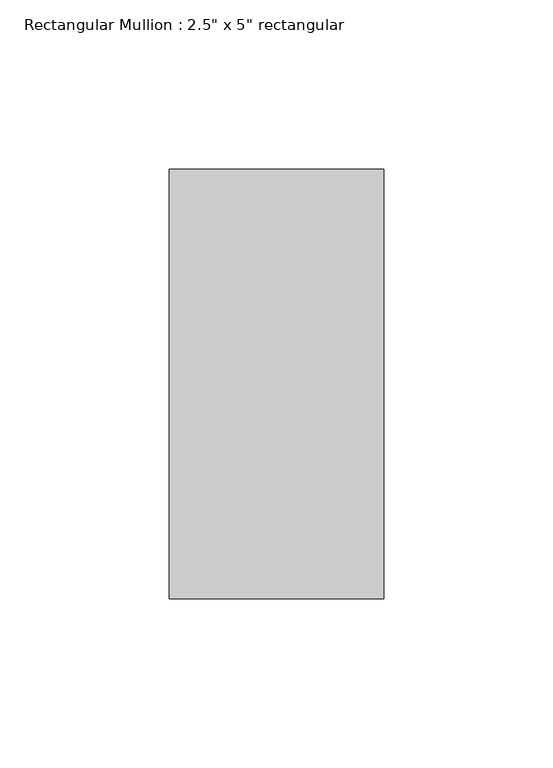
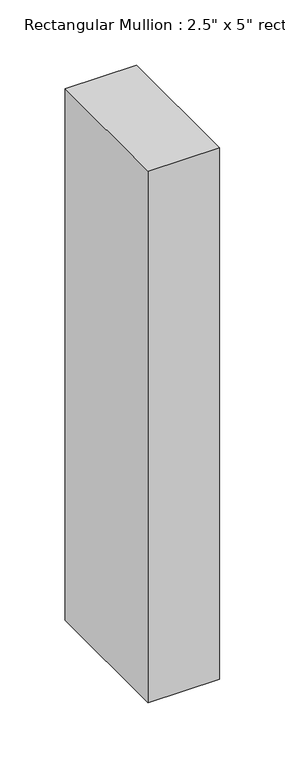
"""IFC4 building model written with IfcOpenShell, lengths in millimetres: member geometry."""

from ifc_helpers import new_model, si_unit, frame, origin, place, context, project, spatial, polyline, outline, extrude, source, transform, mapped, element, save


def member_43b2f8c3(model_context):
    return source(origin(), model_context, "Body", "SweptSolid", [
        extrude(outline(polyline([(0.0, 63.5), (0.0, -63.5), (-63.5, -63.5), (-63.5, 63.5), (0.0, 63.5)])), frame((0.0, 0.0, -497.4166667), z_axis=(0.0, 0.0, 1.0), x_axis=(1.0, 0.0, 0.0)), (0.0, 0.0, 1.0), 497.4166667),
    ])


if __name__ == "__main__":
    model = new_model("IFC4")
    model_context = context("Model", 3, world=origin())
    ifc_project = project(units=[si_unit("LENGTHUNIT", "METRE", prefix="MILLI")], contexts=[model_context])
    site = spatial("IfcSite", under=ifc_project)
    building = spatial("IfcBuilding", under=site)
    placement = place(None, origin())
    member_shape = member_43b2f8c3(model_context)
    element("IfcMember", 1, ObjectType="Rectangular Mullion : 2.5\" x 5\" rectangular", at=placement, inside=building, context=model_context, shape_type="MappedRepresentation", body=[
        mapped(member_shape, transform((0.0, 0.0, 0.0), x_axis=(1.0, 0.0, 0.0), y_axis=(0.0, 1.0, 0.0), z_axis=(0.0, 0.0, 1.0))),
    ])
    save(model, "model.ifc")

# Revit data of these elements
# Type "Rectangular Mullion : 2.5\" x 5\" rectangular"
#   built-in parameter 1007304 = 0.416667 (stored number, unit not read)
#   built-in parameter 1007301 = 0.104167 (stored number, unit not read)
#   built-in parameter 1007300 = 0.104167 (stored number, unit not read)
# Element 1 (IfcMember, "Rectangular Mullion : 2.5\" x 5\" rectangular")
#   Materials on its faces: "Aluminum"
# Materials
#   "Aluminum": class "Metal", colour RGB 247 247 247, transparency 0, Description = "Aluminum 6061", Cost = 0
